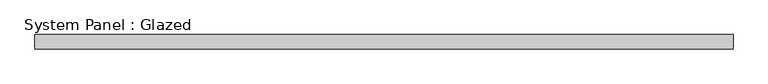
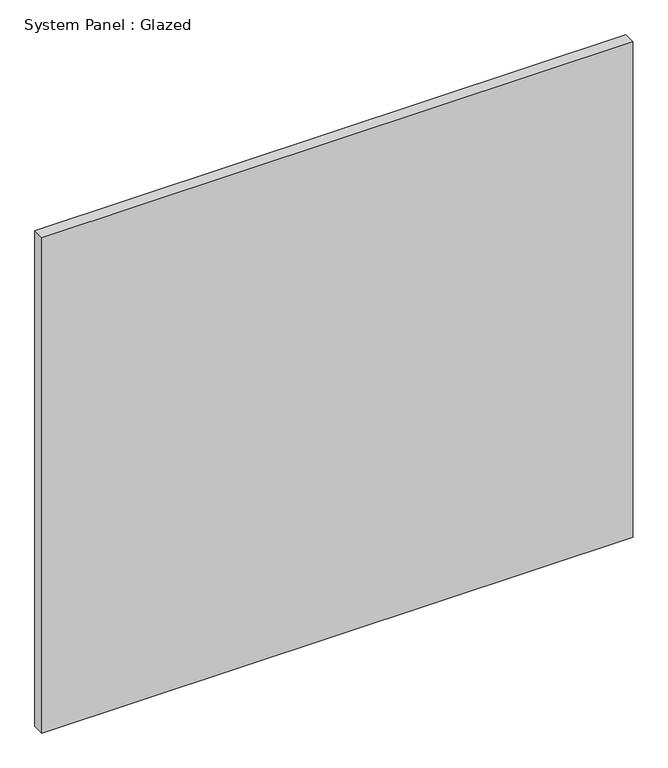
"""IFC4 building model written with IfcOpenShell, lengths in millimetres: plate geometry, System Panel : Glazed."""

from ifc_helpers import new_model, si_unit, origin, origin_with_axes, place, context, project, spatial, polyline, outline, extrude, source, transform, mapped, element, save


def system_panel_glazed_8ae75b46(model_context):
    return source(origin(), model_context, "Body", "SweptSolid", [
        extrude(outline(polyline([(615.95, 19.05), (-615.95, 19.05), (-615.95, 44.45), (615.95, 44.45), (615.95, 19.05)])), origin_with_axes(), (0.0, 0.0, 1.0), 1092.2),
    ])


if __name__ == "__main__":
    model = new_model("IFC4")
    model_context = context("Model", 3, world=origin())
    ifc_project = project(units=[si_unit("LENGTHUNIT", "METRE", prefix="MILLI")], contexts=[model_context])
    site = spatial("IfcSite", under=ifc_project)
    building = spatial("IfcBuilding", under=site)
    placement = place(None, origin())
    system_panel_glazed_shape = system_panel_glazed_8ae75b46(model_context)
    element("IfcPlate", 1, ObjectType="System Panel : Glazed", at=placement, inside=building, context=model_context, shape_type="MappedRepresentation", body=[
        mapped(system_panel_glazed_shape, transform((0.0, 0.0, 0.0), x_axis=(1.0, 0.0, 0.0), y_axis=(0.0, 1.0, 0.0), z_axis=(0.0, 0.0, 1.0))),
    ])
    save(model, "model.ifc")

# Revit data of these elements
# Type "System Panel : Glazed"
#   Construction Type Id = "GSP4R"
#   Analytic Construction = "1/8 in Pilkington single glazing"
#   Visual Light Transmittance = 0.9
#   Solar Heat Gain Coefficient = 0.86
#   Heat Transfer Coefficient (U) = 1.18115 BTU/(h·ft²·°F)
#   Define Thermal Properties by = 1
# Element 1 (IfcPlate, "System Panel : Glazed")
#   Materials on its faces: "Glass"
# Materials
#   "Glass": class "Glass", colour RGB 0 128 192, transparency 0.75, Description = "Soda Lime Glass", Cost = 0
